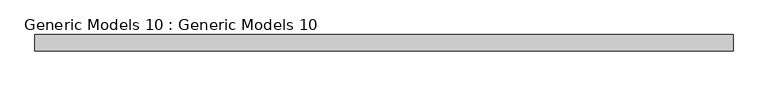
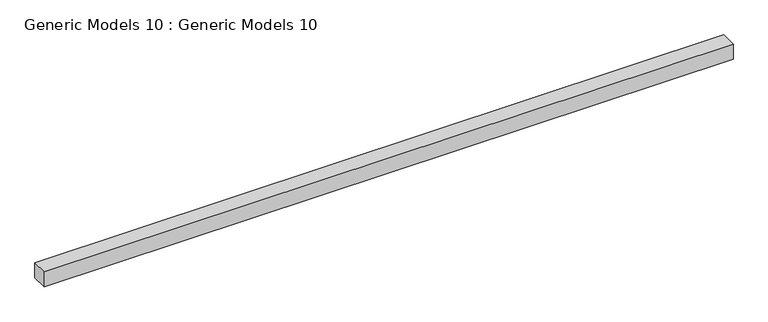
"""IFC4 building model written with IfcOpenShell, lengths in millimetres: proxy geometry, Generic Models 10 : Generic Models 10."""

from ifc_helpers import new_model, si_unit, frame, origin, place, context, project, spatial, polyline, outline, extrude, source, transform, mapped, element, save


def generic_models_10_generic_models_10_b1b5e2eb(model_context):
    return source(origin(), model_context, "Body", "SweptSolid", [
        extrude(outline(polyline([(-2636.9482439, -5874.9827462), (-9088.5482439, -5874.9827462), (-9088.5482439, -5722.5827462), (-2636.9482439, -5722.5827462), (-2636.9482439, -5874.9827462)])), frame((0.0, 0.0, 6556.9880505), z_axis=(0.0, 0.0, 1.0), x_axis=(1.0, 0.0, 0.0)), (0.0, 0.0, 1.0), 148.6119495),
    ])


if __name__ == "__main__":
    model = new_model("IFC4")
    model_context = context("Model", 3, world=origin())
    ifc_project = project(units=[si_unit("LENGTHUNIT", "METRE", prefix="MILLI")], contexts=[model_context])
    site = spatial("IfcSite", under=ifc_project)
    building = spatial("IfcBuilding", under=site)
    placement = place(None, origin())
    generic_models_10_generic_models_10_shape = generic_models_10_generic_models_10_b1b5e2eb(model_context)
    element("IfcBuildingElementProxy", 1, Name="Generic Models 10 : Generic Models 10", ObjectType="Generic Models 10 : Generic Models 10", at=placement, inside=building, context=model_context, shape_type="MappedRepresentation", body=[
        mapped(generic_models_10_generic_models_10_shape, transform((0.0, 0.0, 0.0), x_axis=(1.0, 0.0, 0.0), y_axis=(0.0, 1.0, 0.0), z_axis=(0.0, 0.0, 1.0))),
    ])
    save(model, "model.ifc")

# Revit data of these elements
# Element 1 (IfcBuildingElementProxy, "Generic Models 10 : Generic Models 10")
#   Materials on its faces: "GLASS MATERIAL"
# Materials
#   "GLASS MATERIAL": class "Generic", colour RGB 120 120 120, transparency 0, Cost = 0
